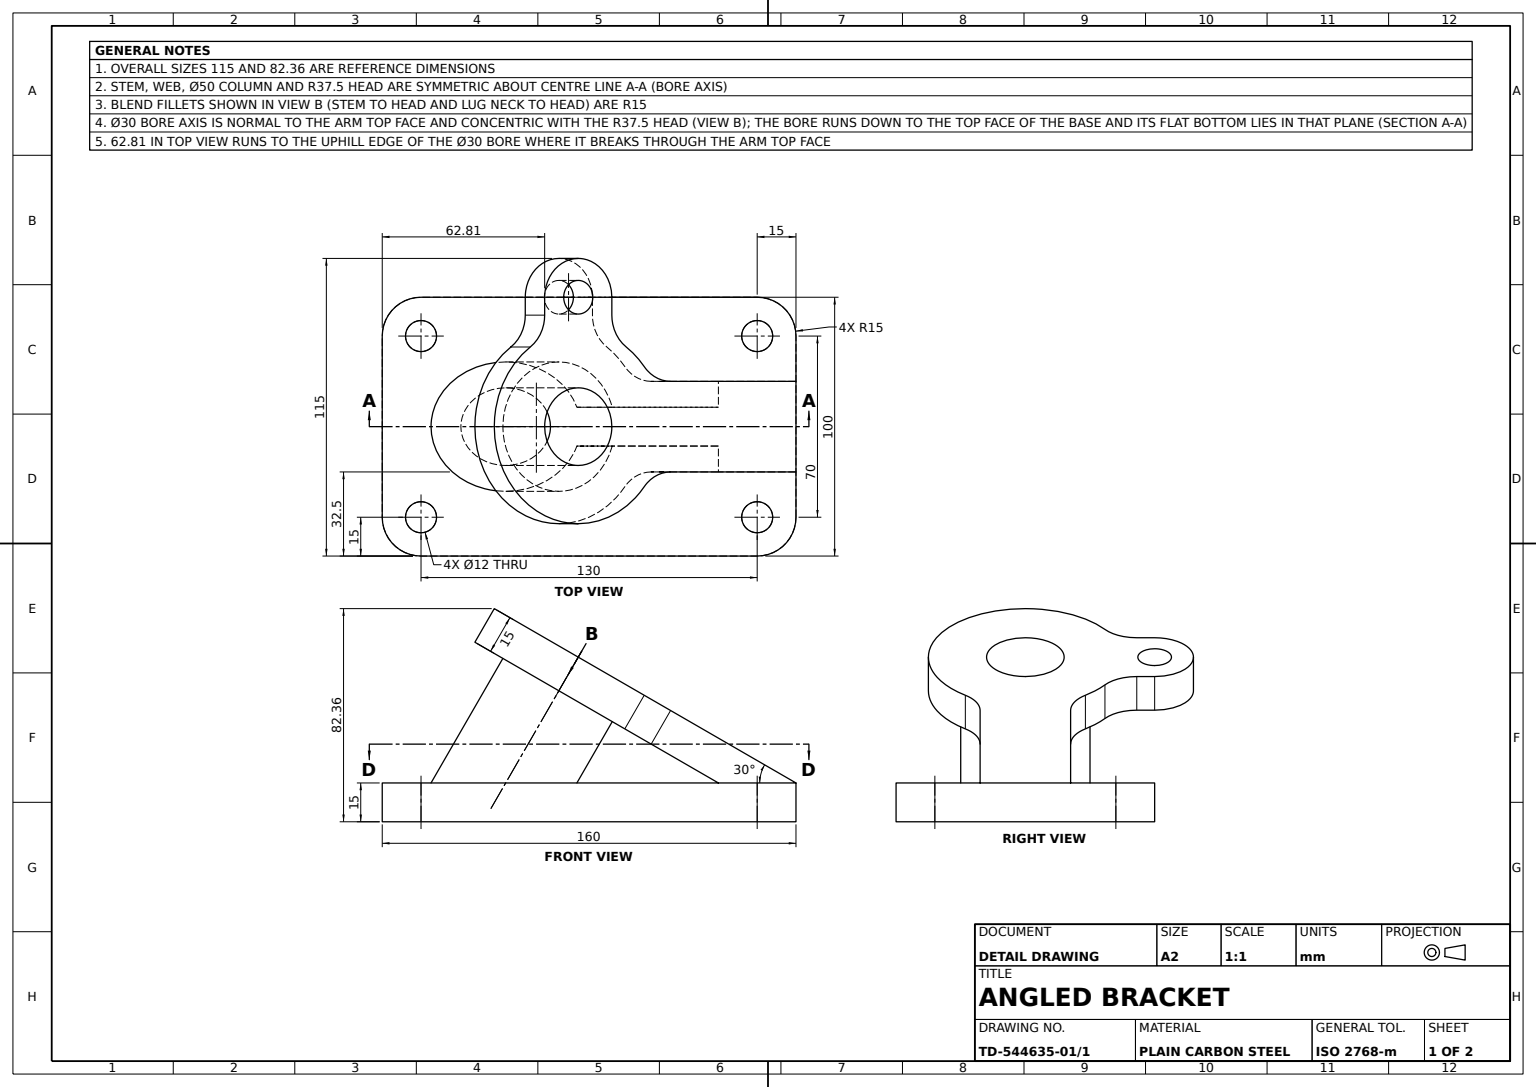
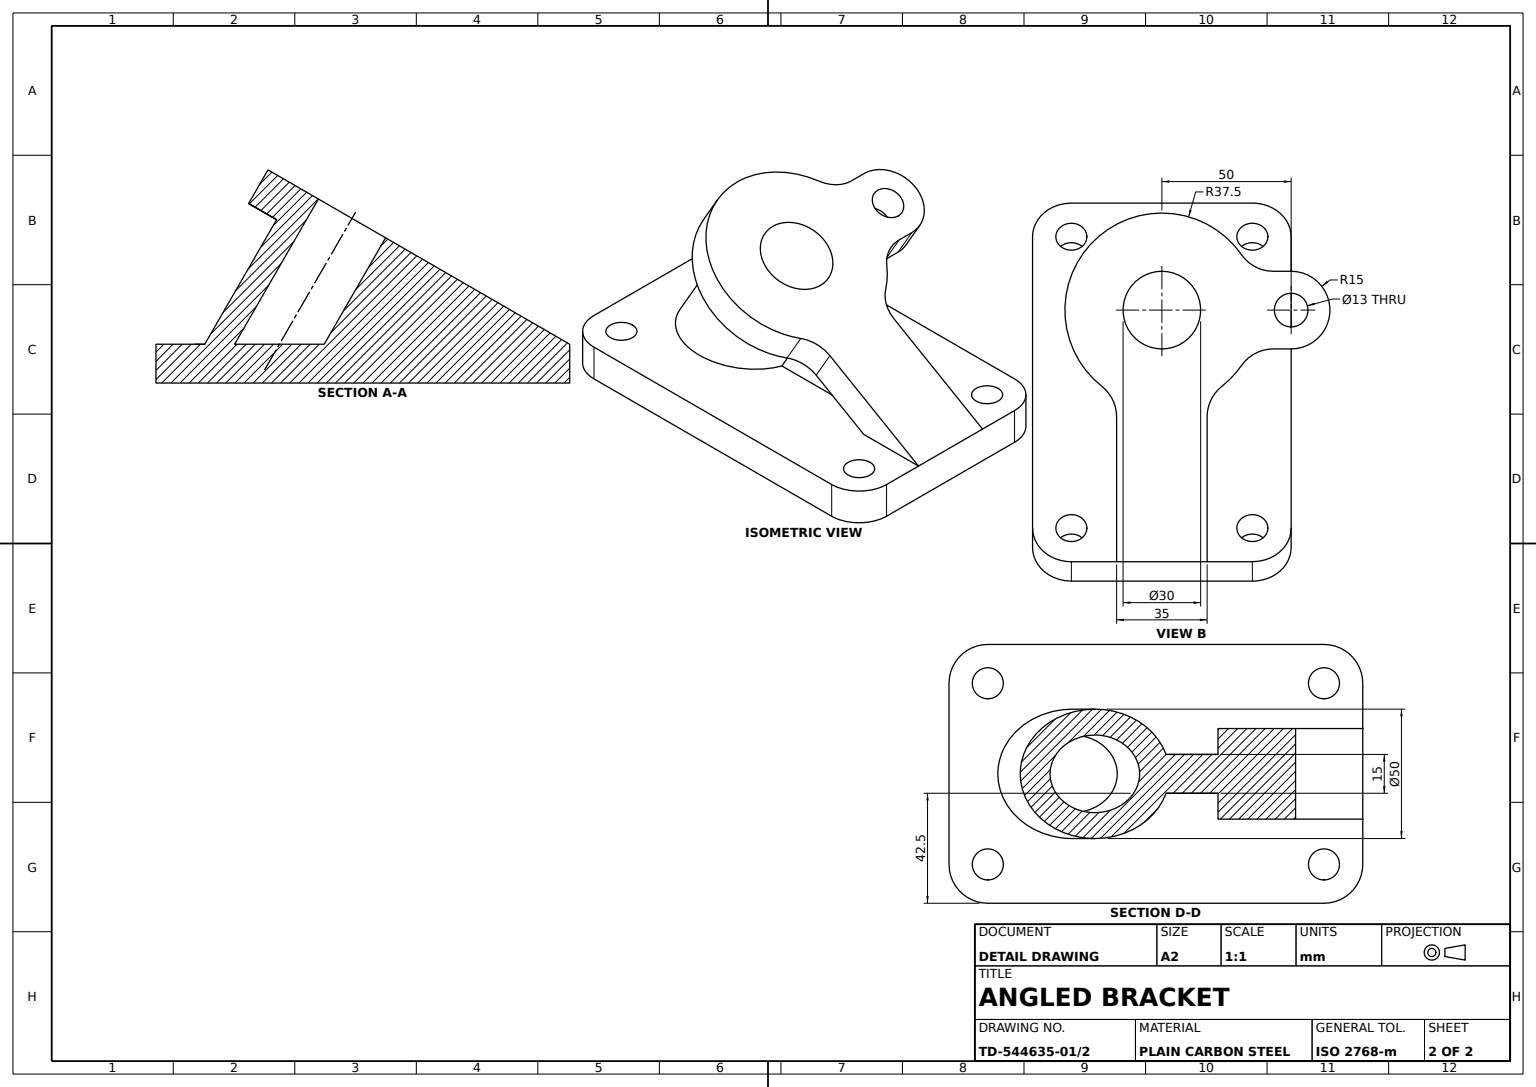
from build123d import *

# Parameters (mm, degrees)
BASE_PLATE_SKETCH_W             = 160
BASE_PLATE_SKETCH_H             = 100
BASE_PLATE_160X100X15_DEPTH     = 15
BASE_PLATE_CORNER_FILLETS_R15_R = 15
MOUNTING_HOLES_SKETCH_R         = 6
MOUNTING_HOLES_4X_12_DEPTH      = 15
INCLINED_ARM_PROFILE_SKETCH_R   = 15
INCLINED_ARM_PROFILE_SKETCH_R_2 = 6.5
INCLINED_ARM_DEPTH              = 15
ARM_SUPPORT_WEB_REACH           = 134.937
ARM_SUPPORT_WEB_SKETCH_R        = 15


with BuildPart() as part:
    # Base Plate Sketch → Base Plate 160x100x15 (new body)
    with BuildSketch(Plane(origin=(0, 0, 0), x_dir=(1, 0, 0), z_dir=(0, 1, 0))):
        Rectangle(BASE_PLATE_SKETCH_W, BASE_PLATE_SKETCH_H)
    extrude(amount=BASE_PLATE_160X100X15_DEPTH)

    # Base Plate Corner Fillets R15
    base_plate_corner_fillets_r15_edges = [part.edges().sort_by_distance(p)[0] for p in [
        (80, 7.5, 50),
        (-80, 7.5, 50),
        (-80, 7.5, -50),
        (80, 7.5, -50),
    ]]
    fillet(base_plate_corner_fillets_r15_edges, radius=BASE_PLATE_CORNER_FILLETS_R15_R)

    # Mounting Holes Sketch → Mounting Holes 4x_12 (cut)
    with BuildSketch(Plane(origin=(0, 15, 0), x_dir=(1, 0, 0), z_dir=(0, 1, 0))):
        with Locations(Location((-65, 35, 0), (0, 0, 270))):
            Circle(MOUNTING_HOLES_SKETCH_R)
        with Locations(Location((65, 35, 0), (0, 0, 270))):
            Circle(MOUNTING_HOLES_SKETCH_R)
        with Locations(Location((65, -35, 0), (0, 0, 270))):
            Circle(MOUNTING_HOLES_SKETCH_R)
        with Locations(Location((-65, -35, 0), (0, 0, 270))):
            Circle(MOUNTING_HOLES_SKETCH_R)
    extrude(amount=-MOUNTING_HOLES_4X_12_DEPTH, mode=Mode.SUBTRACT)

    # Arm Support Web: up to this face of the body (flat: up to its plane)
    arm_support_web_end = Plane(part.part.faces().sort_by_distance((0, 15, 0))[0])
    # Arm Support Web Sketch → Arm Support Web (add, up to the picked face)
    with BuildSketch(Plane(origin=(26.495190528, 45.891016151, 0), x_dir=(0.8660254037844417, -0.4999999999999947, 0), z_dir=(0.4999999999999947, 0.8660254037844417, 0)), mode=Mode.PRIVATE) as arm_support_web_sk1:
        with BuildLine():
            Line((61.782032303, 7.5), (61.782032303, -7.5))
            Line((61.782032303, -7.5), (-11.591402841, -7.5))
            ThreePointArc((-11.591402841, -7.5), (-60.439882876, 0), (-11.591402841, 7.5))
            Line((-11.591402841, 7.5), (61.782032303, 7.5))
        make_face()
        with Locations(Location((-35.439882876, 0, 0), (0, 0, 180))):
            Circle(ARM_SUPPORT_WEB_SKETCH_R, mode=Mode.SUBTRACT)
    arm_support_web_tool1 = split(extrude(arm_support_web_sk1.sketch, amount=-ARM_SUPPORT_WEB_REACH, mode=Mode.PRIVATE), bisect_by=arm_support_web_end, keep=Keep.BOTH, mode=Mode.PRIVATE)


with BuildPart() as body_2:
    # Inclined Arm Profile Sketch → Inclined Arm (new body)
    with BuildSketch(Plane(origin=(26.495190528, 45.891016151, 0), x_dir=(-0.8660254037844417, 0.4999999999999947, 0), z_dir=(0.4999999999999947, 0.8660254037844417, 0))):
        with BuildLine():
            Line((-61.782032303, -17.5), (-5.79117338, -17.5))
            ThreePointArc((-5.79117338, -17.5), (0.755363327, -19.003968837), (5.989128407, -23.214285714))
            ThreePointArc((5.989128407, -23.214285714), (9.720912357, -27.290741204), (14.011311447, -30.774442749))
            ThreePointArc((14.011311447, -30.774442749), (18.735961782, -36.140569101), (20.439882876, -43.084219849))
            Line((20.439882876, -43.084219849), (20.439882876, -50))
            ThreePointArc((20.439882876, -50), (35.439882876, -65), (50.439882876, -50))
            Line((50.439882876, -50), (50.439882876, -43.084219849))
            ThreePointArc((50.439882876, -43.084219849), (52.14380397, -36.140569101), (56.868454305, -30.774442749))
            ThreePointArc((56.868454305, -30.774442749), (62.73062408, 25.718970519), (5.989128407, 23.214285714))
            ThreePointArc((5.989128407, 23.214285714), (0.755363327, 19.003968837), (-5.79117338, 17.5))
            Line((-5.79117338, 17.5), (-61.782032303, 17.5))
            Line((-61.782032303, 17.5), (-61.782032303, -17.5))
        make_face()
        with Locations((35.439882876, 0)):
            Circle(INCLINED_ARM_PROFILE_SKETCH_R, mode=Mode.SUBTRACT)
        with Locations((35.439882876, -50)):
            Circle(INCLINED_ARM_PROFILE_SKETCH_R_2, mode=Mode.SUBTRACT)
    extrude(amount=-INCLINED_ARM_DEPTH)


with BuildPart() as part_1:
    add(part.part)

    add(body_2.part)  # Arm Support Web merges body 2
    add(arm_support_web_tool1.solids().sort_by(Axis((20.297634, 49.469177, 0), (-0.4999999999999947, -0.8660254037844417, 0)))[0])


solid = part_1.part
